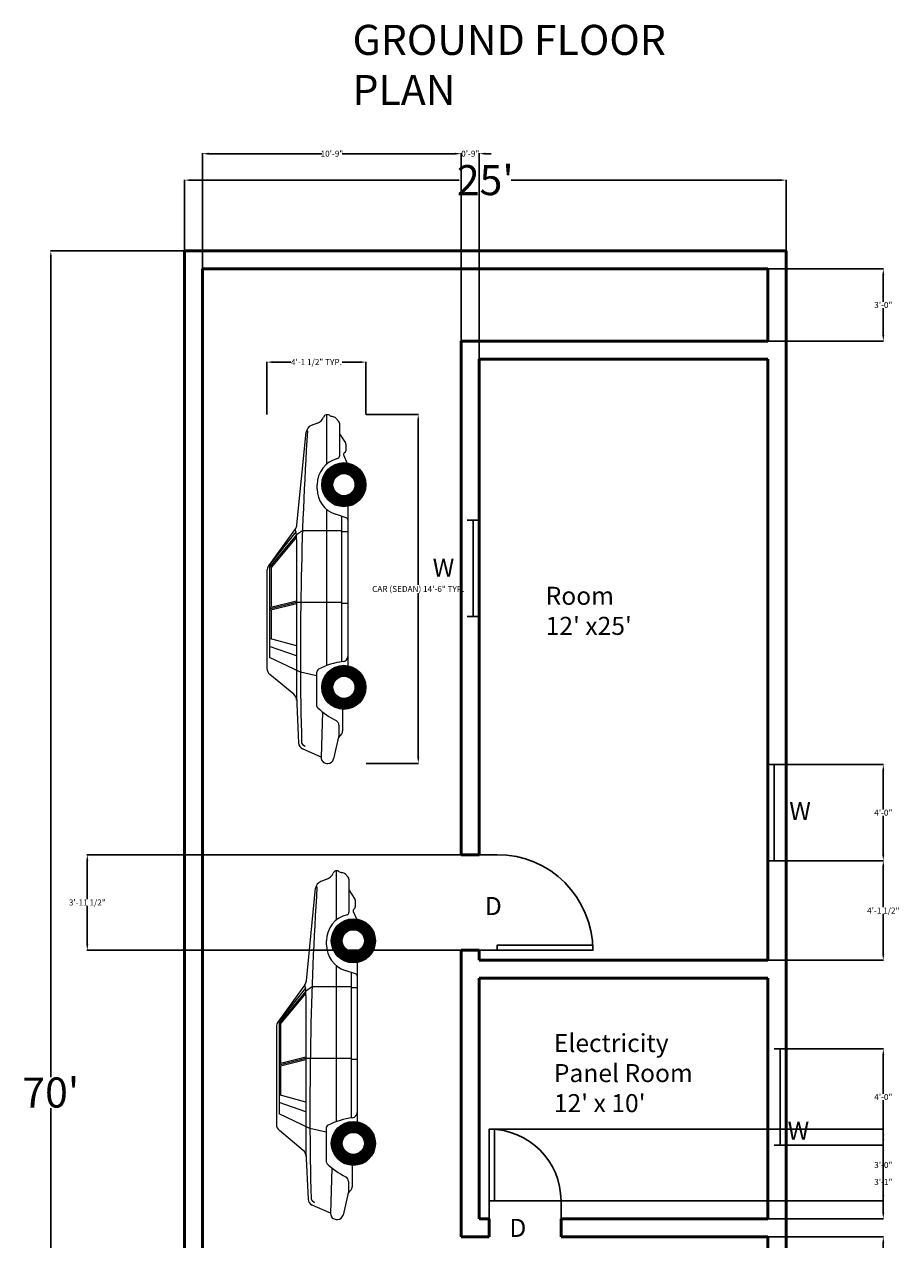
# Model space of a CAD drawing. Units: inches. Extents: x -250 to 2650, y 180 to 1183.
# Tile 3 of 10: x -250 to 186, y 577 to 1183. Entities that reach past the tile are written whole.
import ezdxf

# ---------------------------------------------------------------- set-up
doc = ezdxf.new("R2010")
doc.units = ezdxf.units.IN
doc.header["$MEASUREMENT"] = 0
for name, color, linetype, lineweight in [('A-ANNO-DIMS', 2, 'Continuous', 18), ('A-ANNO-TEXT', 7, 'Continuous', 18), ('A-AREA-IDEN', 3, 'Continuous', 18), ('A-DOOR', 4, 'Continuous', 25), ('A-EQPM', 8, 'Continuous', 18), ('A-GLAZ', 3, 'Continuous', 25), ('A-WALL', 7, 'Continuous', 50)]:
    doc.layers.add(name, color=color, linetype=linetype, lineweight=lineweight)
doc.styles.get("Standard").update_dxf_attribs({"font": 'arial.ttf'})
doc.dimstyles.get("Standard").update_dxf_attribs({"dimtxt": 3, "dimasz": 3, "dimexe": 0.18, "dimexo": 0.0625, "dimgap": 0.09, "dimtad": 0, "dimtih": 1, "dimtoh": 1, "dimdec": 0, "dimzin": 0, "dimdsep": 46, "dimlunit": 3, "dimtxsty": 'Standard', "dimcen": 0.09, "dimadec": 0, "dimazin": 0, "dimtfac": 1, "dimtdec": 0, "dimtofl": 0, "dimtmove": 0, "dimatfit": 3, "dimfxl": 1, "dimtolj": 1, "dimtzin": 0, "dimarcsym": 0})

# ---------------------------------------------------------------- blocks, each defined once
blk = doc.blocks.new('*U5')
for p, q in [((-48, 6), (-48, 0)), ((0, 3), (-48, 3)), ((0, 6), (0, 0))]:
    blk.add_line(p, q)
blk = doc.blocks.new('*U6')
for p, q in [((-48, 6), (-48, 0)), ((0, 3), (-48, 3)), ((0, 6), (0, 0))]:
    blk.add_line(p, q)
blk = doc.blocks.new('*U9')
for p, q in [((0, 0), (0, -6)), ((24, 0), (24, -6))]:
    blk.add_line(p, q)
blk.add_lwpolyline([(0, 0), (0, 24), (1.75, 24), (1.75, 0)], close=True)
blk.add_arc((0, 0), 24, 0, 90)
blk = doc.blocks.new('*U10')
for p, q in [((-32, 0), (-32, -6)), ((0, 0), (0, -6))]:
    blk.add_line(p, q)
blk.add_lwpolyline([(0, 0), (0, 32), (-1.75, 32), (-1.75, 0)], close=True)
blk.add_arc((0, 0), 32, 90, 180)
blk = doc.blocks.new('Car - sedan  side')
for p, q in [((-77.81, 49.34), (-126.58, 49.34)), ((-56.87, 35.13), (-75.48, 48.59)), ((-139.53, 35.99), (-129.64, 47.91)), ((-128.57, 32.64), (-121.22, 48.02)), ((-74.7, 48.02), (-121.22, 48.02)), ((-120.32, 34.67), (-115.67, 48.02)), ((-115.4, 34.67), (-111.74, 48.02)), ((-97.55, 47.3), (-111.94, 47.3)), ((-94.41, 34.67), (-97.73, 48.02)), ((-93.72, 34.67), (-97.04, 48.02)), ((-93.03, 34.67), (-96.34, 48.02)), ((-76.26, 47.3), (-96.16, 47.3)), ((-61.08, 34.66), (-76.26, 47.3)), ((-60.02, 34.65), (-76.07, 48.02)), ((-58.54, 34.93), (-74.99, 48.02)), ((-170.93, 22.32), (-166.81, 31.56)), ((-164.57, 31.6), (-165.48, 30.35)), ((-140.23, 34.67), (-163.88, 33.56)), ((-62.28, 34.67), (-140.23, 34.67)), ((-130.39, 24.63), (-128.57, 32.64)), ((-93.72, 19.62), (-93.72, 34.67)), ((-62.28, 34.67), (-60.02, 34.65)), ((-60.02, 34.65), (-58.54, 34.93)), ((-57.97, 31.61), (-60.02, 34.65)), ((-57.21, 35.38), (-58.54, 34.93)), ((-57.97, 19.62), (-57.97, 31.61)), ((-54.93, 34.4), (-8.75, 29.8)), ((-128.78, 24.63), (-144.79, 24.63)), ((-36.97, 24.38), (-34.94, 24.38)), ((-4.21, 24.18), (-5.42, 27.27)), ((-174, 19.51), (-174, 18.91)), ((-148.26, 21.7), (-171.11, 22.33)), ((-47.2, 19.62), (-125.23, 19.62)), ((-93.72, 12.14), (-93.72, 19.62)), ((-57.97, 12.14), (-57.97, 19.62)), ((0, 19.62), (-24.7, 19.62)), ((-160.12, 13.48), (-171.81, 16.16)), ((-159.22, 12.14), (-161.08, 13.7)), ((-155.01, 13.48), (-160.12, 13.48)), ((-50.67, 12.14), (-123.32, 12.14)), ((-94.21, 9.03), (-94.21, 12.14)), ((-58.39, 9.03), (-58.39, 12.14)), ((-51.4, 9.89), (-49.69, 15.14)), ((-4.23, 13.19), (-20.72, 13.19)), ((-9.5, 13.19), (-14.1, 10.2)), ((-3.22, 13.59), (-1.77, 14.97)), ((-147.03, 11.6), (-157.73, 11.6)), ((-120.62, 9.03), (-125.23, 9.03)), ((-45.76, 9.03), (-120.62, 9.03)), ((-20.36, 11.06), (-24.06, 9.44)), ((-18.83, 10.42), (-19.11, 10.76)), ((-14.68, 10.03), (-18.01, 10.03))]:
    blk.add_line(p, q)
at = {"const_width": 5.49}
for points in [[(-127.8, 11, -1), (-144.3, 11, -1)], [(-26.69, 11, -1), (-43.19, 11, -1)]]:
    blk.add_lwpolyline(points, format="xyb", close=True, dxfattribs=at)
for centre, radius in [((-136.05, 11), 11), ((-34.94, 11), 11), ((-136.05, 11), 5.51), ((-34.94, 11), 5.51)]:
    blk.add_circle(centre, radius)
for centre, radius, start, end in [((-126.58, 45.38), 3.97, 90, 140.30288), ((-77.81, 45.38), 3.97, 54.13504, 90), ((-163.72, 30.18), 3.38, 92.68266, 155.97362), ((-163.62, 30.91), 1.17, 91.49105, 143.95527), ((-118.51, -1702.12), 1734.79, 86.34698, 91.49105), ((-142.58, 38.53), 3.97, 272.68265, 320.30288), ((-54.54, 38.35), 3.97, 234.13503, 264.31231), ((-144.79, 22.64), 1.98, 90, 136.3964), ((-128.78, 22.64), 1.98, 28.1371, 90), ((-36.97, 11), 13.38, 90, 161.97316), ((-34.94, 11), 13.38, 13.58642, 90), ((-9.15, 25.82), 4, 21.31069, 84.3123), ((-171.18, 19.51), 2.82, 88.41927, 180), ((-171.18, 18.91), 2.82, 180, 257.09053), ((-118.09, -2.78), 38.85, 136.3964, 152.90974), ((-157.14, 7.48), 34.14, 6.51354, 28.1371), ((0.9, 26.18), 5.49, 201.3107, 247.70484), ((-1.92, 19.3), 1.94, 325.37436, 67.70485), ((-157.73, 13.93), 2.32, 230.12913, 270), ((-155.01, 16.1), 2.62, 270, 332.90974), ((-20.72, 14.43), 1.24, 193.58641, 270), ((-4.23, 14.65), 1.46, 270, 313.71735), ((-3.82, 17.12), 2.96, 313.71735, 352.38387), ((2.46, 16.28), 3.37, 145.37437, 172.38386), ((-120.62, 11.65), 2.62, 186.51353, 270), ((-52.58, 10.27), 1.24, 270, 341.97316), ((-19.93, 10.09), 1.06, 39.30103, 113.71592), ((-18.01, 11.09), 1.06, 219.30104, 270), ((-14.68, 11.09), 1.06, 270, 303.04697)]:
    blk.add_arc(centre, radius, start, end)
blk = doc.blocks.new('*D13')
at = {"layer": 'A-ANNO-DIMS', "color": 0, "lineweight": -2, "transparency": 16777216}
for p, q in [((-169.97, 1070.09), (-169.97, 1105.5)), ((-166.97, 1105.32), (-32.92, 1105.32)), ((127.03, 1105.32), (-7.02, 1105.32)), ((130.03, 1070.09), (130.03, 1105.5))]:
    blk.add_line(p, q, dxfattribs=at)
at = {"layer": 'A-ANNO-DIMS', "color": 0, "transparency": 16777216}
for points in [[(-166.97, 1105.82), (-166.97, 1104.82), (-169.97, 1105.32)], [(127.03, 1105.82), (127.03, 1104.82), (130.03, 1105.32)]]:
    blk.add_solid(points, dxfattribs=at)
at = {"layer": 'Defpoints', "color": 0, "transparency": 16777216}
for p in [(-169.97, 1105.32), (-169.97, 1070.02), (130.03, 1070.02)]:
    blk.add_point(p, dxfattribs=at)
at = {"layer": 'A-ANNO-DIMS', "color": 0, "transparency": 16777216, "insert": (-19.97, 1105.32), "char_height": 3, "attachment_point": 5}
blk.add_mtext("\\A1;{\\H5x;25'}", dxfattribs=at)
blk = doc.blocks.new('*D14')
at = {"layer": 'A-ANNO-DIMS', "color": 0, "lineweight": -2, "transparency": 16777216}
for p, q in [((-170.03, 1070.02), (-236.85, 1070.02)), ((-236.67, 1067.02), (-236.67, 657.77)), ((-236.67, 233.02), (-236.67, 642.28)), ((-170.03, 230.02), (-236.85, 230.02))]:
    blk.add_line(p, q, dxfattribs=at)
at = {"layer": 'A-ANNO-DIMS', "color": 0, "transparency": 16777216}
for points in [[(-237.17, 1067.02), (-236.17, 1067.02), (-236.67, 1070.02)], [(-237.17, 233.02), (-236.17, 233.02), (-236.67, 230.02)]]:
    blk.add_solid(points, dxfattribs=at)
at = {"layer": 'Defpoints', "color": 0, "transparency": 16777216}
for p in [(-169.97, 1070.02), (-236.67, 230.02), (-169.97, 230.02)]:
    blk.add_point(p, dxfattribs=at)
at = {"layer": 'A-ANNO-DIMS', "color": 0, "transparency": 16777216, "insert": (-236.67, 650.02), "char_height": 3, "attachment_point": 5}
blk.add_mtext("\\A1;{\\H5x;70'}", dxfattribs=at)
blk = doc.blocks.new('*D50')
at = {"layer": 'A-ANNO-DIMS', "color": 0, "lineweight": -2, "transparency": 16777216}
for p, q in [((-79.45, 988.39), (-53.22, 988.39)), ((-53.4, 985.39), (-53.4, 903.39)), ((-53.4, 817.28), (-53.4, 899.28)), ((-79.45, 814.28), (-53.22, 814.28))]:
    blk.add_line(p, q, dxfattribs=at)
at = {"layer": 'A-ANNO-DIMS', "color": 0, "transparency": 16777216}
for points in [[(-53.9, 985.39), (-52.9, 985.39), (-53.4, 988.39)], [(-53.9, 817.28), (-52.9, 817.28), (-53.4, 814.28)]]:
    blk.add_solid(points, dxfattribs=at)
at = {"layer": 'Defpoints', "color": 0, "transparency": 16777216}
for p in [(-79.51, 988.39), (-53.4, 988.39), (-79.51, 814.28)]:
    blk.add_point(p, dxfattribs=at)
at = {"layer": 'A-ANNO-DIMS', "color": 0, "transparency": 16777216, "insert": (-53.4, 901.33), "char_height": 3, "attachment_point": 5}
blk.add_mtext('\\A1;CAR (SEDAN) 14\'-6" TYP.', dxfattribs=at)
blk = doc.blocks.new('*D51')
at = {"layer": 'A-ANNO-DIMS', "color": 0, "lineweight": -2, "transparency": 16777216}
for p, q in [((-128.86, 988.45), (-128.86, 1014.69)), ((-125.86, 1014.51), (-116.98, 1014.51)), ((-82.51, 1014.51), (-91.4, 1014.51)), ((-79.51, 988.45), (-79.51, 1014.69))]:
    blk.add_line(p, q, dxfattribs=at)
at = {"layer": 'A-ANNO-DIMS', "color": 0, "transparency": 16777216}
for points in [[(-125.86, 1015.01), (-125.86, 1014.01), (-128.86, 1014.51)], [(-82.51, 1015.01), (-82.51, 1014.01), (-79.51, 1014.51)]]:
    blk.add_solid(points, dxfattribs=at)
at = {"layer": 'Defpoints', "color": 0, "transparency": 16777216}
for p in [(-128.86, 1014.51), (-128.86, 988.39), (-79.51, 988.39)]:
    blk.add_point(p, dxfattribs=at)
at = {"layer": 'A-ANNO-DIMS', "color": 0, "transparency": 16777216, "insert": (-104.19, 1014.51), "char_height": 3, "attachment_point": 5}
blk.add_mtext('\\A1;4\'-1 1/2" TYP.', dxfattribs=at)
blk = doc.blocks.new('*D54')
at = {"layer": 'A-ANNO-DIMS', "color": 0, "lineweight": -2, "transparency": 16777216}
for p, q in [((121.09, 1061.02), (178.71, 1061.02)), ((178.53, 1058.02), (178.53, 1044.65)), ((178.53, 1028.02), (178.53, 1041.4)), ((121.09, 1025.02), (178.71, 1025.02))]:
    blk.add_line(p, q, dxfattribs=at)
at = {"layer": 'A-ANNO-DIMS', "color": 0, "transparency": 16777216}
for points in [[(178.03, 1058.02), (179.03, 1058.02), (178.53, 1061.02)], [(178.03, 1028.02), (179.03, 1028.02), (178.53, 1025.02)]]:
    blk.add_solid(points, dxfattribs=at)
at = {"layer": 'Defpoints', "color": 0, "transparency": 16777216}
for p in [(121.03, 1061.02), (178.53, 1061.02), (121.03, 1025.02)]:
    blk.add_point(p, dxfattribs=at)
at = {"layer": 'A-ANNO-DIMS', "color": 0, "transparency": 16777216, "insert": (178.53, 1043.02), "char_height": 3, "attachment_point": 5}
blk.add_mtext('\\A1;3\'-0"', dxfattribs=at)
blk = doc.blocks.new('*D55')
at = {"layer": 'A-ANNO-DIMS', "color": 0, "lineweight": -2, "transparency": 16777216}
for p, q in [((-160.97, 1061.09), (-160.97, 1118.7)), ((-157.97, 1118.52), (-101.57, 1118.52)), ((-34.97, 1118.52), (-91.37, 1118.52)), ((-31.97, 1025.09), (-31.97, 1118.7))]:
    blk.add_line(p, q, dxfattribs=at)
at = {"layer": 'A-ANNO-DIMS', "color": 0, "transparency": 16777216}
for points in [[(-157.97, 1119.02), (-157.97, 1118.02), (-160.97, 1118.52)], [(-34.97, 1119.02), (-34.97, 1118.02), (-31.97, 1118.52)]]:
    blk.add_solid(points, dxfattribs=at)
at = {"layer": 'Defpoints', "color": 0, "transparency": 16777216}
for p in [(-31.97, 1118.52), (-160.97, 1061.02), (-31.97, 1025.02)]:
    blk.add_point(p, dxfattribs=at)
at = {"layer": 'A-ANNO-DIMS', "color": 0, "transparency": 16777216, "insert": (-96.47, 1118.52), "char_height": 3, "attachment_point": 5}
blk.add_mtext('\\A1;10\'-9"', dxfattribs=at)
blk = doc.blocks.new('*D56')
at = {"layer": 'A-ANNO-DIMS', "color": 0, "lineweight": -2, "transparency": 16777216}
for p, q in [((-34.97114, 1118.524548), (-37.97114, 1118.524548)), ((-31.97114, 1025.087048), (-31.97114, 1118.704548)), ((-22.97114, 1016.087048), (-22.97114, 1118.704548)), ((-19.97114, 1118.524548), (-16.97114, 1118.524548))]:
    blk.add_line(p, q, dxfattribs=at)
at = {"layer": 'A-ANNO-DIMS', "color": 0, "transparency": 16777216}
for points in [[(-34.97114, 1119.024548), (-34.97114, 1118.024548), (-31.97114, 1118.524548)], [(-19.97114, 1119.024548), (-19.97114, 1118.024548), (-22.97114, 1118.524548)]]:
    blk.add_solid(points, dxfattribs=at)
at = {"layer": 'Defpoints', "color": 0, "transparency": 16777216}
for p in [(-22.97114, 1118.524548), (-31.97114, 1025.024548), (-22.97114, 1016.024548)]:
    blk.add_point(p, dxfattribs=at)
at = {"layer": 'A-ANNO-DIMS', "color": 0, "transparency": 16777216, "insert": (-27.47114, 1118.524548), "char_height": 3, "attachment_point": 5}
blk.add_mtext('\\A1;0\'-9"', dxfattribs=at)
blk = doc.blocks.new('*D57')
at = {"layer": 'A-ANNO-DIMS', "color": 0, "lineweight": -2, "transparency": 16777216}
for p, q in [((-23.03, 768.72), (-218.65, 768.72)), ((-218.47, 765.72), (-218.47, 746.52)), ((-218.47, 724.02), (-218.47, 743.23)), ((-23.03, 721.02), (-218.65, 721.02))]:
    blk.add_line(p, q, dxfattribs=at)
at = {"layer": 'A-ANNO-DIMS', "color": 0, "transparency": 16777216}
for points in [[(-218.97, 765.72), (-217.97, 765.72), (-218.47, 768.72)], [(-218.97, 724.02), (-217.97, 724.02), (-218.47, 721.02)]]:
    blk.add_solid(points, dxfattribs=at)
at = {"layer": 'Defpoints', "color": 0, "transparency": 16777216}
for p in [(-22.97, 768.72), (-218.47, 721.02), (-22.97, 721.02)]:
    blk.add_point(p, dxfattribs=at)
at = {"layer": 'A-ANNO-DIMS', "color": 0, "transparency": 16777216, "insert": (-218.47, 744.87), "char_height": 3, "attachment_point": 5}
blk.add_mtext('\\A1;3\'-11 1/2"', dxfattribs=at)
blk = doc.blocks.new('*D58')
at = {"layer": 'A-ANNO-DIMS', "color": 0, "lineweight": -2, "transparency": 16777216}
for p, q in [((17.87, 578.02), (178.71, 578.02)), ((178.53, 575.02), (178.53, 410.15)), ((178.53, 242.02), (178.53, 406.9)), ((-160.91, 239.02), (178.71, 239.02))]:
    blk.add_line(p, q, dxfattribs=at)
at = {"layer": 'A-ANNO-DIMS', "color": 0, "transparency": 16777216}
for points in [[(178.03, 575.02), (179.03, 575.02), (178.53, 578.02)], [(178.03, 242.02), (179.03, 242.02), (178.53, 239.02)]]:
    blk.add_solid(points, dxfattribs=at)
at = {"layer": 'Defpoints', "color": 0, "transparency": 16777216}
for p in [(17.8, 578.02), (-160.97, 239.02), (178.53, 239.02)]:
    blk.add_point(p, dxfattribs=at)
at = {"layer": 'A-ANNO-DIMS', "color": 0, "transparency": 16777216, "insert": (178.53, 408.52), "char_height": 3, "attachment_point": 5}
blk.add_mtext('\\A1;28\'-3"', dxfattribs=at)
blk = doc.blocks.new('*D59')
at = {"layer": 'A-ANNO-DIMS', "color": 0, "lineweight": -2, "transparency": 16777216}
for p, q in [((-17.91, 631.74), (178.71, 631.74)), ((178.53, 628.74), (178.53, 615.48)), ((178.53, 598.97), (178.53, 612.23)), ((-17.91, 595.97), (178.71, 595.97))]:
    blk.add_line(p, q, dxfattribs=at)
at = {"layer": 'A-ANNO-DIMS', "color": 0, "transparency": 16777216}
for points in [[(178.03, 628.74), (179.03, 628.74), (178.53, 631.74)], [(178.03, 598.97), (179.03, 598.97), (178.53, 595.97)]]:
    blk.add_solid(points, dxfattribs=at)
at = {"layer": 'Defpoints', "color": 0, "transparency": 16777216}
for p in [(-17.97, 631.74), (178.53, 631.74), (-17.97, 595.97)]:
    blk.add_point(p, dxfattribs=at)
at = {"layer": 'A-ANNO-DIMS', "color": 0, "transparency": 16777216, "insert": (178.53, 613.86), "char_height": 3, "attachment_point": 5}
blk.add_mtext('\\A1;3\'-0"', dxfattribs=at)
blk = doc.blocks.new('*D68')
at = {"layer": 'A-ANNO-DIMS', "color": 0, "lineweight": -2, "transparency": 16777216}
for p, q in [((121.09, 765.68), (178.71, 765.68)), ((178.53, 762.68), (178.53, 742.49)), ((178.53, 719.02), (178.53, 739.21)), ((121.09, 716.02), (178.71, 716.02))]:
    blk.add_line(p, q, dxfattribs=at)
at = {"layer": 'A-ANNO-DIMS', "color": 0, "transparency": 16777216}
for points in [[(178.03, 762.68), (179.03, 762.68), (178.53, 765.68)], [(178.03, 719.02), (179.03, 719.02), (178.53, 716.02)]]:
    blk.add_solid(points, dxfattribs=at)
at = {"layer": 'Defpoints', "color": 0, "transparency": 16777216}
for p in [(121.03, 765.68), (178.53, 765.68), (121.03, 716.02)]:
    blk.add_point(p, dxfattribs=at)
at = {"layer": 'A-ANNO-DIMS', "color": 0, "transparency": 16777216, "insert": (178.53, 740.85), "char_height": 3, "attachment_point": 5}
blk.add_mtext('\\A1;4\'-1 1/2"', dxfattribs=at)
blk = doc.blocks.new('*D69')
at = {"layer": 'A-ANNO-DIMS', "color": 0, "lineweight": -2, "transparency": 16777216}
for p, q in [((121.09, 813.68), (178.71, 813.68)), ((178.53, 810.68), (178.53, 791.3)), ((178.53, 768.68), (178.53, 788.06)), ((121.09, 765.68), (178.71, 765.68))]:
    blk.add_line(p, q, dxfattribs=at)
at = {"layer": 'A-ANNO-DIMS', "color": 0, "transparency": 16777216}
for points in [[(178.03, 810.68), (179.03, 810.68), (178.53, 813.68)], [(178.03, 768.68), (179.03, 768.68), (178.53, 765.68)]]:
    blk.add_solid(points, dxfattribs=at)
at = {"layer": 'Defpoints', "color": 0, "transparency": 16777216}
for p in [(121.03, 813.68), (178.53, 813.68), (121.03, 765.68)]:
    blk.add_point(p, dxfattribs=at)
at = {"layer": 'A-ANNO-DIMS', "color": 0, "transparency": 16777216, "insert": (178.53, 789.68), "char_height": 3, "attachment_point": 5}
blk.add_mtext('\\A1;4\'-0"', dxfattribs=at)
blk = doc.blocks.new('*D70')
at = {"layer": 'A-ANNO-DIMS', "color": 0, "lineweight": -2, "transparency": 16777216}
for p, q in [((124.09, 623.78), (178.71, 623.78)), ((178.53, 620.78), (178.53, 607.02)), ((178.53, 590.02), (178.53, 603.78)), ((121.09, 587.02), (178.71, 587.02))]:
    blk.add_line(p, q, dxfattribs=at)
at = {"layer": 'A-ANNO-DIMS', "color": 0, "transparency": 16777216}
for points in [[(178.03, 620.78), (179.03, 620.78), (178.53, 623.78)], [(178.03, 590.02), (179.03, 590.02), (178.53, 587.02)]]:
    blk.add_solid(points, dxfattribs=at)
at = {"layer": 'Defpoints', "color": 0, "transparency": 16777216}
for p in [(124.03, 623.78), (178.53, 623.78), (121.03, 587.02)]:
    blk.add_point(p, dxfattribs=at)
at = {"layer": 'A-ANNO-DIMS', "color": 0, "transparency": 16777216, "insert": (178.53, 605.4), "char_height": 3, "attachment_point": 5}
blk.add_mtext('\\A1;3\'-1"', dxfattribs=at)
blk = doc.blocks.new('*D71')
at = {"layer": 'A-ANNO-DIMS', "color": 0, "lineweight": -2, "transparency": 16777216}
for p, q in [((124.09, 671.78), (178.71, 671.78)), ((178.53, 668.78), (178.53, 649.4)), ((178.53, 626.78), (178.53, 646.16)), ((124.09, 623.78), (178.71, 623.78))]:
    blk.add_line(p, q, dxfattribs=at)
at = {"layer": 'A-ANNO-DIMS', "color": 0, "transparency": 16777216}
for points in [[(178.03, 668.78), (179.03, 668.78), (178.53, 671.78)], [(178.03, 626.78), (179.03, 626.78), (178.53, 623.78)]]:
    blk.add_solid(points, dxfattribs=at)
at = {"layer": 'Defpoints', "color": 0, "transparency": 16777216}
for p in [(124.03, 671.78), (178.53, 671.78), (124.03, 623.78)]:
    blk.add_point(p, dxfattribs=at)
at = {"layer": 'A-ANNO-DIMS', "color": 0, "transparency": 16777216, "insert": (178.53, 647.78), "char_height": 3, "attachment_point": 5}
blk.add_mtext('\\A1;4\'-0"', dxfattribs=at)

msp = doc.modelspace()

# ---------------------------------------------------------------- linework, layer by layer
at = {"layer": 'A-WALL'}
for p, q in [((130.03, 1070.02), (-169.97, 1070.02)), ((-169.97, 1070.02), (-169.97, 230.02)), ((130.03, 230.02), (130.03, 1070.02)), ((121.03, 1061.02), (-160.97, 1061.02)), ((-160.97, 1061.02), (-160.97, 239.02)), ((121.03, 1025.02), (121.03, 1061.02)), ((-31.97, 768.72), (-31.97, 1025.02)), ((121.03, 1025.02), (-31.97, 1025.02)), ((-22.97, 768.72), (-22.97, 1016.02)), ((121.03, 1016.02), (-22.97, 1016.02)), ((121.03, 716.02), (121.03, 1016.02)), ((-22.97, 768.72), (-31.97, 768.72)), ((-31.97, 578.02), (-31.97, 721.02)), ((-22.97, 721.02), (-31.97, 721.02)), ((-22.97, 716.02), (-22.97, 721.02)), ((121.03, 716.02), (-22.97, 716.02)), ((-22.97, 587.02), (-22.97, 707.02)), ((121.03, 707.02), (-22.97, 707.02)), ((121.03, 587.02), (121.03, 707.02)), ((-22.97, 587.02), (-17.97, 587.02)), ((-17.97, 587.02), (-17.97, 578.02)), ((121.03, 587.02), (17.8, 587.02)), ((17.8, 587.02), (17.8, 578.02)), ((-17.97, 578.02), (-31.97, 578.02)), ((121.03, 578.02), (17.8, 578.02)), ((121.03, 332.02), (121.03, 578.02))]:
    msp.add_line(p, q, dxfattribs=at)

# ---------------------------------------------------------------- block references
at = {"layer": 'A-DOOR', "xscale": 1.490620935821662, "yscale": 1.490620935821662, "zscale": 1.490620935821662, "rotation": 270}
msp.add_blockref('*U10', (-14.03, 721.02), dxfattribs=at)
at = {"layer": 'A-DOOR', "xscale": 1.490620935821662, "yscale": 1.490620935821662, "zscale": 1.490620935821662}
msp.add_blockref('*U9', (-17.97, 595.97), dxfattribs=at)
at = {"layer": 'A-EQPM', "rotation": 90}
for p in [(-79.51, 988.28), (-74.77, 760.69)]:
    msp.add_blockref('Car - sedan  side', p, dxfattribs=at)
at = {"layer": 'A-GLAZ', "rotation": 270}
for name, p in [('*U5', (-28.97, 887.58)), ('*U5', (121.03, 765.68)), ('*U6', (124.03, 623.78))]:
    msp.add_blockref(name, p, dxfattribs=at)

# ---------------------------------------------------------------- texts
at = {"layer": 'A-ANNO-TEXT', "attachment_point": 1}
for s, width, insert, char_height in [('GROUND FLOOR PLAN ', 207.4062, (-86.17, 1182.82), 15), ('W', 44.7265, (-46.21, 916.41), 9), ('W', 44.7265, (131.63, 795.06), 9), ('D', 44.7265, (-20.2, 747.58), 9), ('W', 44.7265, (130.8, 635.47), 9), ('D', 44.7265, (-7.95, 586.97), 9)]:
    msp.add_mtext_dynamic_manual_height_columns(s, width=width, gutter_width=1, heights=[0], dxfattribs=dict(at, insert=insert, char_height=char_height))
at = {"layer": 'A-AREA-IDEN', "char_height": 9, "attachment_point": 1}
for s, insert in [("Room\\P12' x25'", (10.15, 902.4)), ("Electricity Panel Room 12' x 10'", (14.24, 679.23))]:
    msp.add_mtext_dynamic_manual_height_columns(s, width=87.4783, gutter_width=1, heights=[0], dxfattribs=dict(at, insert=insert))

# ---------------------------------------------------------------- dimensions: what is measured, and where the dimension line sits
at = {"layer": 'A-ANNO-DIMS'}
for base, p1, p2, picture, middle in [((-31.97, 1118.52), (-160.97, 1061.02), (-31.97, 1025.02), '*D55', (-96.47, 1118.52)), ((-22.97, 1118.52), (-31.97, 1025.02), (-22.97, 1016.02), '*D56', (-27.47, 1118.52))]:
    dim = msp.add_linear_dim(base=base, p1=p1, p2=p2, dimstyle='Standard', override={"dimdec": 1, "dimlfac": 1, "dimrnd": 0, "dimzin": 1, "dimdsep": 46, "dimlunit": 4, "dimfrac": 2}, dxfattribs=at)
    dim.commit()
    dim.dimension.update_dxf_attribs({"geometry": picture, "text_midpoint": middle})
dim = msp.add_linear_dim(base=(-169.97, 1105.32), p1=(130.03, 1070.02), p2=(-169.97, 1070.02), text='{\\H5x;<>}', dimstyle='Standard', override={"dimclrd": 0, "dimclre": 0, "dimclrt": 0}, dxfattribs=at)
dim.commit()
dim.dimension.update_dxf_attribs({"geometry": '*D13', "text_midpoint": (-19.97, 1105.32)})
for base, p1, p2, angle, text, override, picture, middle in [((-236.67, 230.02), (-169.97, 1070.02), (-169.97, 230.02), 90, '{\\H5x;<>}', {"dimclrd": 0, "dimclre": 0, "dimclrt": 0}, '*D14', (-236.67, 650.02)), ((-128.8593, 1014.5075), (-79.5144, 988.3904), (-128.8593, 988.3904), 180, '<> TYP.', {"dimdec": 1, "dimrnd": 0, "dimzin": 1, "dimlunit": 4, "dimfrac": 2}, '*D51', (-104.1868, 1014.5075)), ((-53.4, 988.39), (-79.51, 814.28), (-79.51, 988.39), 90, 'CAR (SEDAN) <> TYP.', {"dimdec": 1, "dimrnd": 0, "dimzin": 1, "dimlunit": 4, "dimfrac": 2}, '*D50', (-53.4, 901.33))]:
    dim = msp.add_linear_dim(base=base, p1=p1, p2=p2, angle=angle, text=text, dimstyle='Standard', override=override, dxfattribs=at)
    dim.commit()
    dim.dimension.update_dxf_attribs({"geometry": picture, "text_midpoint": middle})
for base, p1, p2, picture, middle in [((178.53, 1061.02), (121.03, 1025.02), (121.03, 1061.02), '*D54', (178.53, 1043.02)), ((178.53, 813.68), (121.03, 765.68), (121.03, 813.68), '*D69', (178.53, 789.68)), ((-218.47, 721.02), (-22.97, 768.72), (-22.97, 721.02), '*D57', (-218.47, 744.87)), ((178.53, 765.68), (121.03, 716.02), (121.03, 765.68), '*D68', (178.53, 740.85)), ((178.53, 671.78), (124.03, 623.78), (124.03, 671.78), '*D71', (178.53, 647.78)), ((178.53, 631.74), (-17.97, 595.97), (-17.97, 631.74), '*D59', (178.53, 613.86)), ((178.53, 623.78), (121.03, 587.02), (124.03, 623.78), '*D70', (178.53, 605.4)), ((178.53, 239.02), (17.8, 578.02), (-160.97, 239.02), '*D58', (178.53, 408.52))]:
    dim = msp.add_linear_dim(base=base, p1=p1, p2=p2, angle=90, dimstyle='Standard', override={"dimdec": 1, "dimlfac": 1, "dimrnd": 0, "dimzin": 1, "dimdsep": 46, "dimlunit": 4, "dimfrac": 2}, dxfattribs=at)
    dim.commit()
    dim.dimension.update_dxf_attribs({"geometry": picture, "text_midpoint": middle})

doc.saveas('drawing.dxf')
